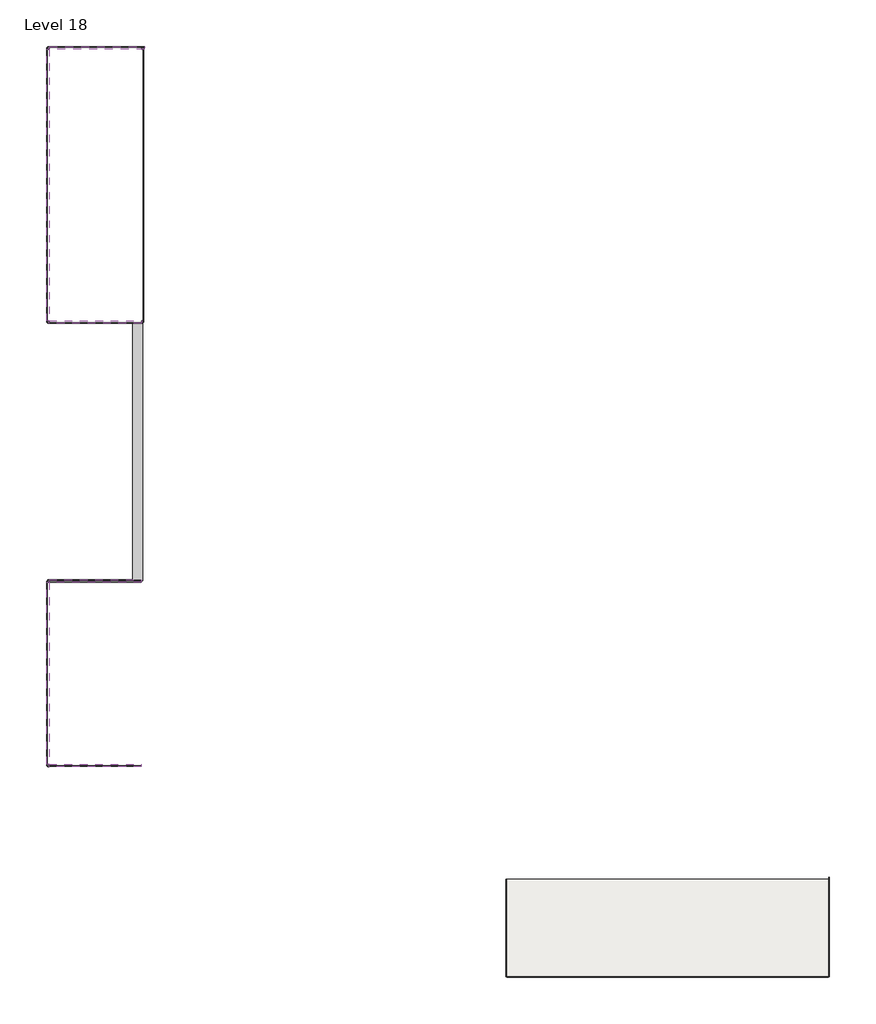
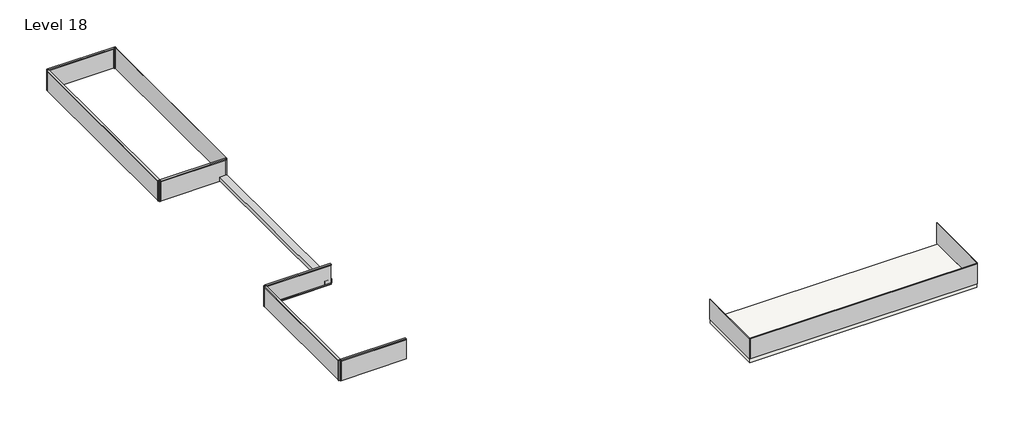
# One storey: 17 members, 10 plates, 1 proxy, 1 slab.
"""IFC4 building model written with IfcOpenShell, lengths in millimetres."""

from ifc_helpers import new_model, si_unit, frame, origin, place, context, project, spatial, polyline, outline, extrude, transform, mapped, element, save
from components import generic_models_15_generic_models_15_8aebc9bb, member_a0ba9e48, member_4491d118, member_6d14b308, member_e7df1716, member_4960e788, member_4d280e20, system_panel_glazed_6303489a, system_panel_glazed_dbf8c7ac, system_panel_glazed_e45de85a, system_panel_glazed_1f759628, system_panel_glazed_f332d308, system_panel_glazed_82bc3a22, system_panel_glazed_9c6e7784, system_panel_glazed_1f6fd899, system_panel_glazed_648d5b1a, system_panel_glazed_42f91ed4

model = new_model("IFC4")

# Units and contexts
model_context = context("Model", 3, world=origin())
ifc_project = project(units=[si_unit("LENGTHUNIT", "METRE", prefix="MILLI")], contexts=[model_context])

# Site, building, storey
site = spatial("IfcSite", under=ifc_project)
building = spatial("IfcBuilding", under=site)
storey = spatial("IfcBuildingStorey", under=building, Name="Level 18", Elevation=29565.6)

# Proxy
placement = place(None, origin())
generic_models_15_generic_models_15_shape = generic_models_15_generic_models_15_8aebc9bb(model_context)
element("IfcBuildingElementProxy", 1, Name="Generic Models 15 : Generic Models 15", ObjectType="Generic Models 15 : Generic Models 15", at=placement, inside=storey, context=model_context, shape_type="MappedRepresentation", body=[
    mapped(generic_models_15_generic_models_15_shape, transform((0.0, 0.0, 0.0), x_axis=(1.0, 0.0, 0.0), y_axis=(0.0, 1.0, 0.0), z_axis=(0.0, 0.0, 1.0))),
])

# Members
member_shape = member_a0ba9e48(model_context)
element("IfcMember", 2, ObjectType="Rectangular Mullion : 2.5\" x 5\" rectangular", at=placement, inside=storey, context=model_context, shape_type="MappedRepresentation", body=[
    mapped(member_shape, transform((-15175.038074, 20810.2014639, 31089.6), x_axis=(0.0, 0.0, 1.0), y_axis=(0.0, -1.0, 0.0), z_axis=(1.0, 0.0, 0.0))),
])
member_2_shape = member_4491d118(model_context)
element("IfcMember", 3, ObjectType="Rectangular Mullion : 2.5\" x 5\" rectangular", at=placement, inside=storey, context=model_context, shape_type="MappedRepresentation", body=[
    mapped(member_2_shape, transform((-20051.838074, 7032.4307139, 29565.6), x_axis=(-1.0, 0.0, 0.0), y_axis=(0.0, 1.0, 0.0), z_axis=(0.0, 0.0, -1.0))),
])
element("IfcMember", 4, ObjectType="Rectangular Mullion : 2.5\" x 5\" rectangular", at=placement, inside=storey, context=model_context, shape_type="MappedRepresentation", body=[
    mapped(member_2_shape, transform((-20051.838074, 20810.2014639, 29565.6), x_axis=(0.0, 1.0, 0.0), y_axis=(1.0, 0.0, 0.0), z_axis=(0.0, 0.0, -1.0))),
])
element("IfcMember", 5, ObjectType="Rectangular Mullion : 2.5\" x 5\" rectangular", at=placement, inside=storey, context=model_context, shape_type="MappedRepresentation", body=[
    mapped(member_2_shape, transform((-20051.838074, -15231.4713044, 29565.6), x_axis=(-1.0, 0.0, 0.0), y_axis=(0.0, 1.0, 0.0), z_axis=(0.0, 0.0, -1.0))),
])
element("IfcMember", 6, ObjectType="Rectangular Mullion : 2.5\" x 5\" rectangular", at=placement, inside=storey, context=model_context, shape_type="MappedRepresentation", body=[
    mapped(member_2_shape, transform((-20051.838074, -5966.8213044, 29565.6), x_axis=(0.0, 1.0, 0.0), y_axis=(1.0, 0.0, 0.0), z_axis=(0.0, 0.0, -1.0))),
])
element("IfcMember", 7, ObjectType="Rectangular Mullion : 2.5\" x 5\" rectangular", at=placement, inside=storey, context=model_context, shape_type="MappedRepresentation", body=[
    mapped(member_2_shape, transform((-20051.838074, 7032.4307139, 31089.6), x_axis=(0.0, -1.0, 0.0), y_axis=(1.0, 0.0, 0.0), z_axis=(0.0, 0.0, 1.0))),
])
element("IfcMember", 8, ObjectType="Rectangular Mullion : 2.5\" x 5\" rectangular", at=placement, inside=storey, context=model_context, shape_type="MappedRepresentation", body=[
    mapped(member_2_shape, transform((-15276.638074, 7032.4307139, 31089.6), x_axis=(1.0, 0.0, 0.0), y_axis=(0.0, 1.0, 0.0), z_axis=(0.0, 0.0, 1.0))),
])
element("IfcMember", 9, ObjectType="Rectangular Mullion : 2.5\" x 5\" rectangular", at=placement, inside=storey, context=model_context, shape_type="MappedRepresentation", body=[
    mapped(member_2_shape, transform((-20051.838074, 20810.2014639, 31089.6), x_axis=(-1.0, 0.0, 0.0), y_axis=(0.0, -1.0, 0.0), z_axis=(0.0, 0.0, 1.0))),
])
element("IfcMember", 10, ObjectType="Rectangular Mullion : 2.5\" x 5\" rectangular", at=placement, inside=storey, context=model_context, shape_type="MappedRepresentation", body=[
    mapped(member_2_shape, transform((-20051.838074, -15231.4713044, 31089.6), x_axis=(0.0, -1.0, 0.0), y_axis=(1.0, 0.0, 0.0), z_axis=(0.0, 0.0, 1.0))),
])
member_3_shape = member_6d14b308(model_context)
element("IfcMember", 11, ObjectType="Rectangular Mullion : 2.5\" x 5\" rectangular", at=placement, inside=storey, context=model_context, shape_type="MappedRepresentation", body=[
    mapped(member_3_shape, transform((-19988.338074, 7032.4307139, 31089.6), x_axis=(0.0, 0.0, 1.0), y_axis=(0.0, 1.0, 0.0), z_axis=(-1.0, 0.0, 0.0))),
])
member_4_shape = member_e7df1716(model_context)
element("IfcMember", 12, ObjectType="Rectangular Mullion : 2.5\" x 5\" rectangular", at=placement, inside=storey, context=model_context, shape_type="MappedRepresentation", body=[
    mapped(member_4_shape, transform((-20051.838074, 20746.7014639, 31089.6), x_axis=(0.0, 0.0, 1.0), y_axis=(1.0, 0.0, 0.0), z_axis=(0.0, 1.0, 0.0))),
])
element("IfcMember", 13, ObjectType="Rectangular Mullion : 2.5\" x 5\" rectangular", at=placement, inside=storey, context=model_context, shape_type="MappedRepresentation", body=[
    mapped(member_2_shape, transform((-15276.638074, 20810.2014639, 31089.6), x_axis=(0.0, 1.0, 0.0), y_axis=(-1.0, 0.0, 0.0), z_axis=(0.0, 0.0, 1.0))),
])
element("IfcMember", 14, ObjectType="Rectangular Mullion : 2.5\" x 5\" rectangular", at=placement, inside=storey, context=model_context, shape_type="MappedRepresentation", body=[
    mapped(member_2_shape, transform((-20051.838074, -5966.8213044, 31089.6), x_axis=(-1.0, 0.0, 0.0), y_axis=(0.0, -1.0, 0.0), z_axis=(0.0, 0.0, 1.0))),
])
member_5_shape = member_4960e788(model_context)
element("IfcMember", 15, ObjectType="Rectangular Mullion : 2.5\" x 5\" rectangular", at=placement, inside=storey, context=model_context, shape_type="MappedRepresentation", body=[
    mapped(member_5_shape, transform((-20051.838074, -6030.3213044, 31089.6), x_axis=(0.0, 0.0, 1.0), y_axis=(1.0, 0.0, 0.0), z_axis=(0.0, 1.0, 0.0))),
])
member_6_shape = member_4d280e20(model_context)
element("IfcMember", 16, ObjectType="Rectangular Mullion : 2.5\" x 5\" rectangular", at=placement, inside=storey, context=model_context, shape_type="MappedRepresentation", body=[
    mapped(member_6_shape, transform((-19988.338074, -15231.4713044, 31089.6), x_axis=(0.0, 0.0, 1.0), y_axis=(0.0, 1.0, 0.0), z_axis=(-1.0, 0.0, 0.0))),
])
element("IfcMember", 17, ObjectType="Rectangular Mullion : 2.5\" x 5\" rectangular", at=placement, inside=storey, context=model_context, shape_type="MappedRepresentation", body=[
    mapped(member_6_shape, transform((-19988.338074, -5966.8213044, 29565.6), x_axis=(0.0, 0.0, -1.0), y_axis=(0.0, -1.0, 0.0), z_axis=(-1.0, 0.0, 0.0))),
])
element("IfcMember", 18, ObjectType="Rectangular Mullion : 2.5\" x 5\" rectangular", at=placement, inside=storey, context=model_context, shape_type="MappedRepresentation", body=[
    mapped(member_6_shape, transform((-15352.838074, -5966.8213044, 31089.6), x_axis=(0.0, 0.0, 1.0), y_axis=(0.0, -1.0, 0.0), z_axis=(1.0, 0.0, 0.0))),
])

# Plates
system_panel_glazed_shape = system_panel_glazed_6303489a(model_context)
element("IfcPlate", 19, ObjectType="System Panel : Glazed", at=placement, inside=storey, context=model_context, shape_type="MappedRepresentation", body=[
    mapped(system_panel_glazed_shape, transform((3011.361926, -23389.9670305, 29565.6), x_axis=(0.0, 1.0, 0.0), y_axis=(-1.0, 0.0, 0.0), z_axis=(0.0, 0.0, 1.0))),
])
system_panel_glazed_2_shape = system_panel_glazed_dbf8c7ac(model_context)
element("IfcPlate", 20, ObjectType="System Panel : Glazed", at=placement, inside=storey, context=model_context, shape_type="MappedRepresentation", body=[
    mapped(system_panel_glazed_2_shape, transform((11088.561926, -25828.3670305, 29565.6), x_axis=(-1.0, 0.0, 0.0), y_axis=(0.0, -1.0, 0.0), z_axis=(0.0, 0.0, 1.0))),
])
system_panel_glazed_3_shape = system_panel_glazed_e45de85a(model_context)
element("IfcPlate", 21, ObjectType="System Panel : Glazed", at=placement, inside=storey, context=model_context, shape_type="MappedRepresentation", body=[
    mapped(system_panel_glazed_3_shape, transform((19165.761926, -23337.0827833, 29565.6), x_axis=(0.0, -1.0, 0.0), y_axis=(1.0, 0.0, 0.0), z_axis=(0.0, 0.0, 1.0))),
])
system_panel_glazed_4_shape = system_panel_glazed_1f759628(model_context)
element("IfcPlate", 22, ObjectType="System Panel : Glazed", at=placement, inside=storey, context=model_context, shape_type="MappedRepresentation", body=[
    mapped(system_panel_glazed_4_shape, transform((-17664.238074, 7032.4307139, 29565.6), x_axis=(-1.0, 0.0, 0.0), y_axis=(0.0, -1.0, 0.0), z_axis=(0.0, 0.0, 1.0))),
])
system_panel_glazed_5_shape = system_panel_glazed_f332d308(model_context)
element("IfcPlate", 23, ObjectType="System Panel : Glazed", at=placement, inside=storey, context=model_context, shape_type="MappedRepresentation", body=[
    mapped(system_panel_glazed_5_shape, transform((-20051.838074, 13921.3160889, 29565.6), x_axis=(0.0, 1.0, 0.0), y_axis=(-1.0, 0.0, 0.0), z_axis=(0.0, 0.0, 1.0))),
])
system_panel_glazed_6_shape = system_panel_glazed_82bc3a22(model_context)
element("IfcPlate", 24, ObjectType="System Panel : Glazed", at=placement, inside=storey, context=model_context, shape_type="MappedRepresentation", body=[
    mapped(system_panel_glazed_6_shape, transform((-17581.688074, 20810.2014639, 29565.6), x_axis=(1.0, 0.0, 0.0), y_axis=(0.0, 1.0, 0.0), z_axis=(0.0, 0.0, 1.0))),
])
system_panel_glazed_7_shape = system_panel_glazed_9c6e7784(model_context)
element("IfcPlate", 25, ObjectType="System Panel : Glazed", at=placement, inside=storey, context=model_context, shape_type="MappedRepresentation", body=[
    mapped(system_panel_glazed_7_shape, transform((-15276.638074, 13889.5660889, 29565.6), x_axis=(0.0, -1.0, 0.0), y_axis=(1.0, 0.0, 0.0), z_axis=(0.0, 0.0, 1.0))),
])
system_panel_glazed_8_shape = system_panel_glazed_1f6fd899(model_context)
element("IfcPlate", 26, ObjectType="System Panel : Glazed", at=placement, inside=storey, context=model_context, shape_type="MappedRepresentation", body=[
    mapped(system_panel_glazed_8_shape, transform((-20051.838074, -10599.1463044, 29565.6), x_axis=(0.0, 1.0, 0.0), y_axis=(-1.0, 0.0, 0.0), z_axis=(0.0, 0.0, 1.0))),
])
system_panel_glazed_9_shape = system_panel_glazed_648d5b1a(model_context)
element("IfcPlate", 27, ObjectType="System Panel : Glazed", at=placement, inside=storey, context=model_context, shape_type="MappedRepresentation", body=[
    mapped(system_panel_glazed_9_shape, transform((-17670.588074, -15231.4713044, 29565.6), x_axis=(-1.0, 0.0, 0.0), y_axis=(0.0, -1.0, 0.0), z_axis=(0.0, 0.0, 1.0))),
])
system_panel_glazed_10_shape = system_panel_glazed_42f91ed4(model_context)
element("IfcPlate", 28, ObjectType="System Panel : Glazed", at=placement, inside=storey, context=model_context, shape_type="MappedRepresentation", body=[
    mapped(system_panel_glazed_10_shape, transform((-17670.588074, -5966.8213044, 29629.1), x_axis=(1.0, 0.0, 0.0), y_axis=(0.0, 1.0, 0.0), z_axis=(0.0, 0.0, 1.0))),
])

# Slab
element("IfcSlab", 29, ObjectType="Generic - 12\"", at=placement, inside=storey, context=model_context, shape_type="SweptSolid", body=[
    extrude(outline(polyline([(3011.361926, -20951.5670305), (19165.761926, -20951.5670305), (19165.761926, -25828.3670305), (3011.361926, -25828.3670305), (3011.361926, -20951.5670305)])), frame((0.0, 0.0, 29260.8), z_axis=(0.0, 0.0, 1.0), x_axis=(1.0, 0.0, 0.0)), (0.0, 0.0, 1.0), 304.8),
])

save(model, "model.ifc")

# Revit data of these elements
# Type "Rectangular Mullion : 2.5\" x 5\" rectangular"
#   built-in parameter 1007304 = 0.416667 (stored number, unit not read)
#   built-in parameter 1007301 = 0.104167 (stored number, unit not read)
#   built-in parameter 1007300 = 0.104167 (stored number, unit not read)
# Type "System Panel : Glazed"
#   Construction Type Id = "GSP4R"
#   Analytic Construction = "1/8 in Pilkington single glazing"
#   Visual Light Transmittance = 0.9
#   Solar Heat Gain Coefficient = 0.86
#   Heat Transfer Coefficient (U) = 1.18115 BTU/(h·ft²·°F)
# Type "Generic - 12\""
#   Assembly Code = "B1010"
#   Function = 0
#   Layers, outside or top first: 1' - 0" no material (function 1)
# Element 1 (IfcBuildingElementProxy, "Generic Models 15 : Generic Models 15")
#   Phase Created = New Construction
# Elements 2, 3, 4, 5, 6, 7, 8, 9, 10, 11, 12, 13, 14, 15, 16, 17, 18 (IfcMember, "Rectangular Mullion : 2.5\" x 5\" rectangular")
#   Phase Created = New Construction
#   Materials on its faces: "Aluminum"
# Elements 19, 20, 21, 22, 23, 24, 25, 26, 27, 28 (IfcPlate, "System Panel : Glazed")
#   Phase Created = New Construction
#   Materials on its faces: "Glass"
# Element 29 (IfcSlab, "Generic - 12\"")
#   built-in parameter 1001955 = 3.14159 (stored number, unit not read)
#   Height Offset From Level = 0' - 0"
#   Phase Created = New Construction
#   Materials on its faces: "Default Floor"
# Materials
#   "Aluminum": class "Metal", colour RGB 247 247 247, transparency 0, Description = "Aluminum 6061", Cost = 0
#   "Glass": class "Glass", colour RGB 0 128 192, transparency 0.75, Description = "Soda Lime Glass", Cost = 0
#   "Default Floor": colour RGB 128 128 128, transparency 0
